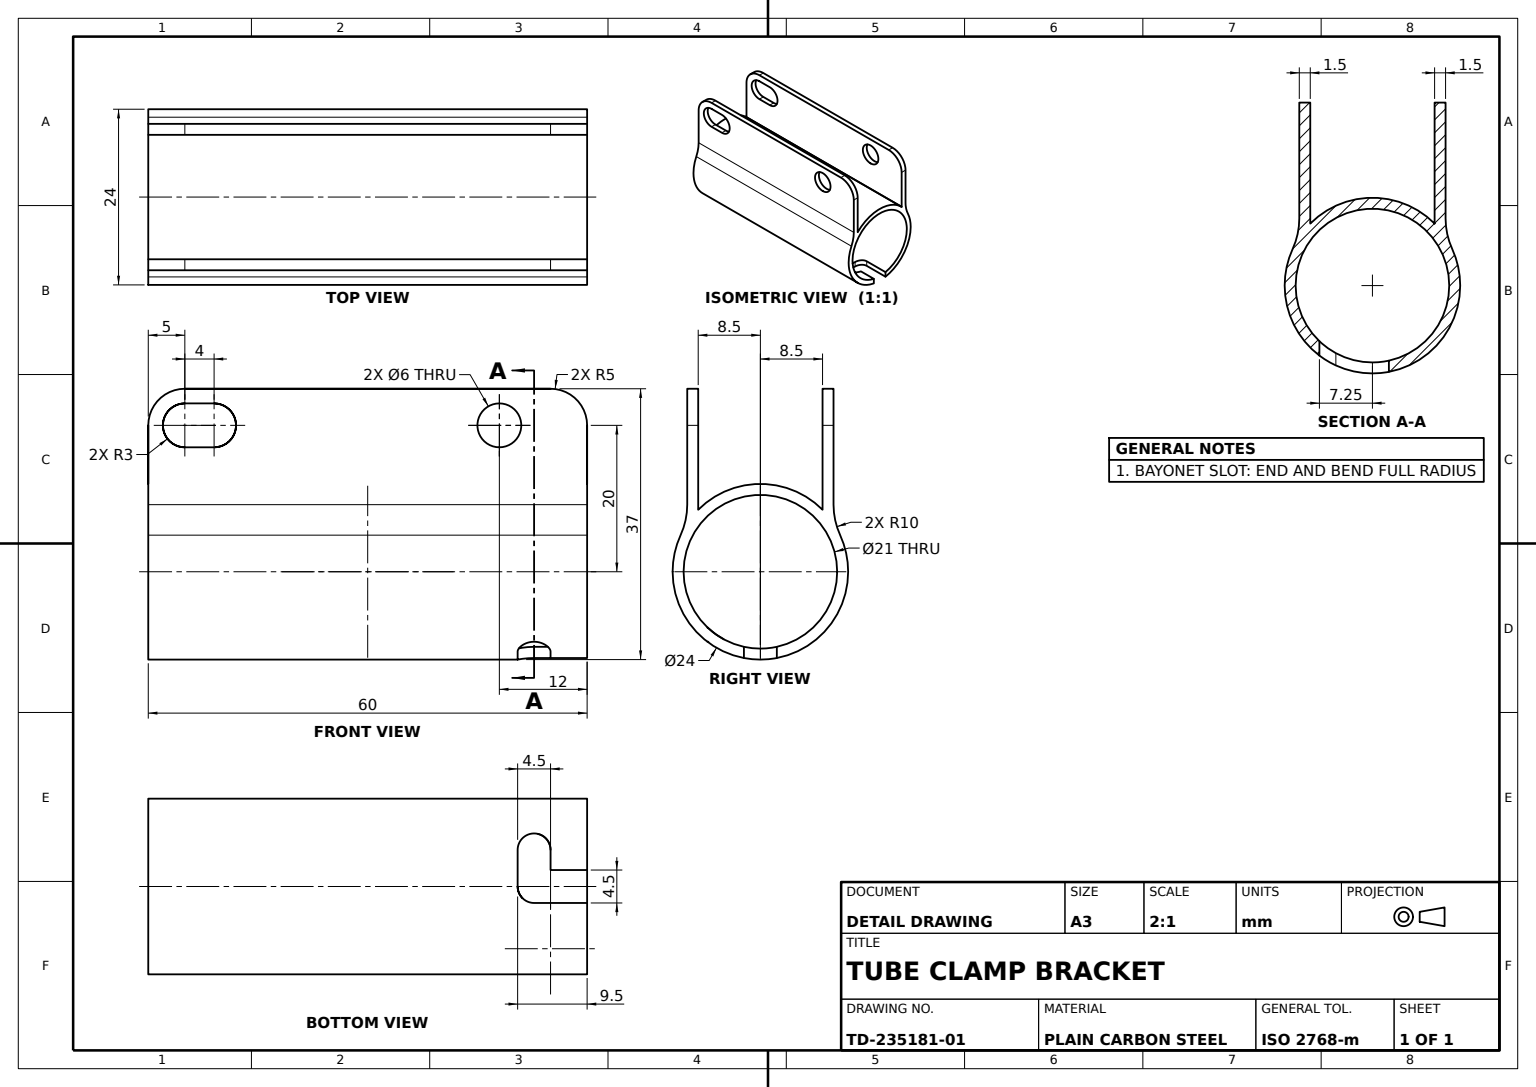
from build123d import *

# Parameters (mm, degrees)
SLEEVE_TUBE_PROFILE_R   = 12
SLEEVE_TUBE_PROFILE_R_2 = 10.5
SLEEVE_TUBE_24X60_DEPTH = 30
MOUNTING_LUGS_DEPTH     = 60
LUG_FILLET_R10_R        = 10
LUG_FILLET_R5_R         = 5
LUG_GAP_CUT_PROFILE_R   = 3
LUG_GAP_CUT_DEPTH       = 60
LUG_SLOTS_REACH         = 42.853
LUG_SLOTS_END_RADIUS    = 12


with BuildPart() as part:
    # Sleeve Tube Profile → Sleeve Tube Ø24x60 (new, symmetric)
    with BuildSketch(Plane.XY):
        Circle(SLEEVE_TUBE_PROFILE_R)
        Circle(SLEEVE_TUBE_PROFILE_R_2, mode=Mode.SUBTRACT)
    extrude(amount=SLEEVE_TUBE_24X60_DEPTH, both=True)

    # Mounting Lugs Profile → Mounting Lugs (add)
    with BuildSketch(Plane.XY.offset(30)):
        with BuildLine():
            Line((-8.5, 25), (-8.5, 8.470537173))
            ThreePointArc((-8.5, 8.470537173), (-9.295504635, 7.589044312), (-10, 6.633249581))
            Line((-10, 6.633249581), (-10, 25))
            Line((-10, 25), (-8.5, 25))
        make_face()
        with BuildLine():
            Line((10, 25), (10, 6.633249581))
            ThreePointArc((10, 6.633249581), (9.295504635, 7.589044312), (8.5, 8.470537173))
            Line((8.5, 8.470537173), (8.5, 25))
            Line((8.5, 25), (10, 25))
        make_face()
    extrude(amount=-MOUNTING_LUGS_DEPTH)

    # Lug Fillet R10
    lug_fillet_r10_edges = [part.edges().sort_by_distance(p)[0] for p in [
        (-10, 6.633249581, 0),
        (10, 6.633249581, 0),
    ]]
    fillet(lug_fillet_r10_edges, radius=LUG_FILLET_R10_R)

    # Lug Fillet R5
    lug_fillet_r5_edges = [part.edges().sort_by_distance(p)[0] for p in [
        (-9.25, 25, -30),
        (-9.25, 25, 30),
        (9.25, 25, -30),
        (9.25, 25, 30),
    ]]
    fillet(lug_fillet_r5_edges, radius=LUG_FILLET_R5_R)

    # Lug Gap Cut Profile → Lug Gap Cut (cut)
    with BuildSketch(Plane(origin=(10, 0, 0), x_dir=(0, 0, -1), z_dir=(1, 0, 0))):
        with Locations(Location((18, 20, 0), (0, 0, 90))):
            Circle(LUG_GAP_CUT_PROFILE_R)
        with BuildLine():
            Line((-25, 23), (-21, 23))
            ThreePointArc((-21, 23), (-18, 20), (-21, 17))
            Line((-21, 17), (-25, 17))
            ThreePointArc((-25, 17), (-28, 20), (-25, 23))
        make_face()
    extrude(amount=-LUG_GAP_CUT_DEPTH, mode=Mode.SUBTRACT)

    # Lug Slots: up to this cylinder (the profile starts inside it)
    lug_slots_end = Plane(origin=(0, 0, -24.504673), z_dir=(0, 0, -1)) * Cylinder(LUG_SLOTS_END_RADIUS, 110.706, mode=Mode.PRIVATE)
    # Lug Slots Profile → Lug Slots (cut, up to the surface)
    with BuildSketch(Plane(origin=(0, 0, 0), x_dir=(1, 0, 0), z_dir=(0, 1, 0)), mode=Mode.PRIVATE) as lug_slots_sk1:
        with BuildLine():
            Line((-2.25, 30), (-2.25, 22.75))
            ThreePointArc((-2.25, 22.75), (-1.590990258, 21.159009742), (0, 20.5))
            Line((0, 20.5), (5, 20.5))
            ThreePointArc((5, 20.5), (7.25, 22.75), (5, 25))
            Line((5, 25), (2.25, 25))
            Line((2.25, 25), (2.25, 30))
            Line((2.25, 30), (-2.25, 30))
        make_face()
    lug_slots_tool1 = extrude(lug_slots_sk1.sketch, amount=-LUG_SLOTS_REACH, mode=Mode.PRIVATE) & lug_slots_end
    add(lug_slots_tool1.solids().sort_by_distance((1.518168, 0, -24.504673))[0], mode=Mode.SUBTRACT)


solid = part.part
